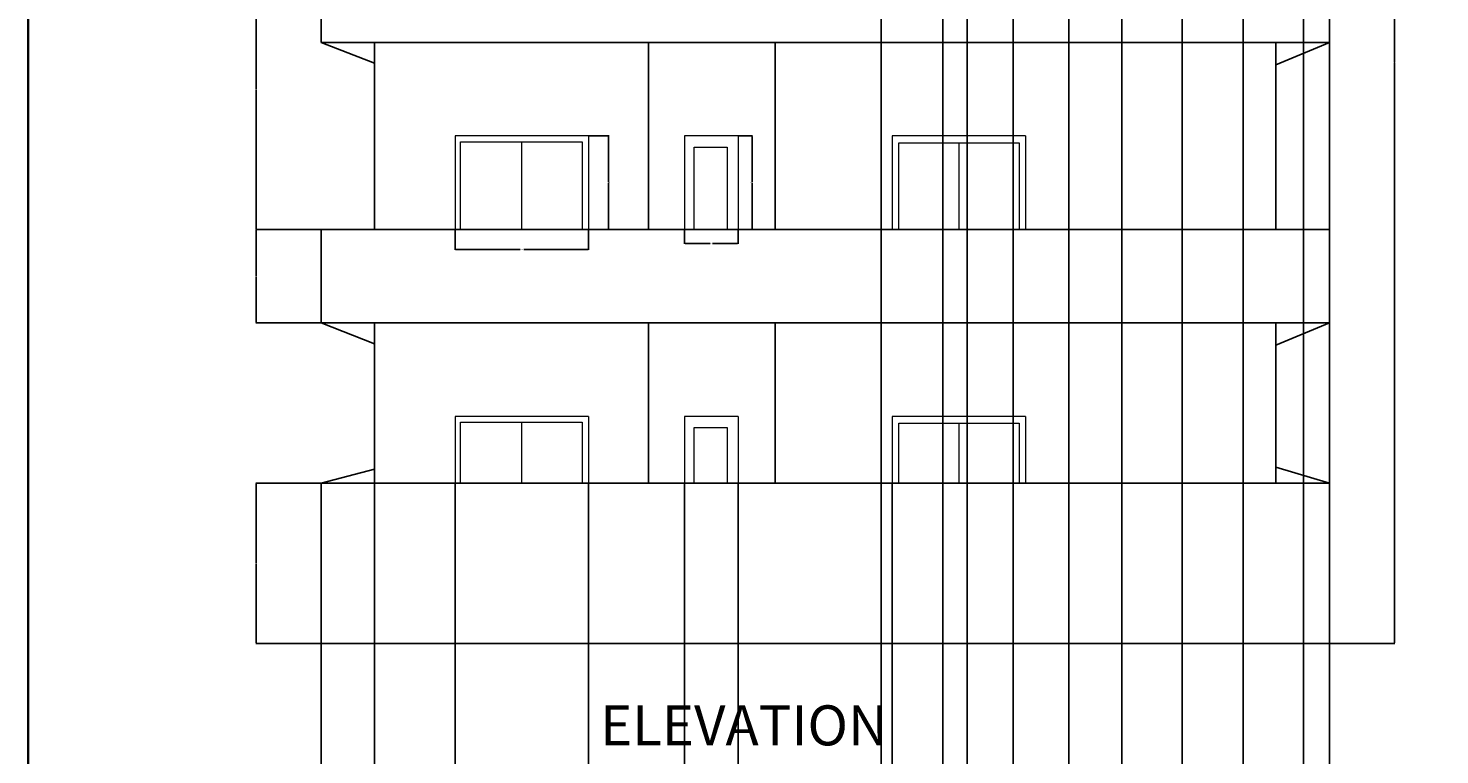
# Model space of a CAD drawing. Units: inches. Extents: x 1955 to 3324, y 980 to 3129.
# Tile 9 of 11: x 1955 to 2589, y 2488 to 2815. Entities that reach past the tile are written whole.
import ezdxf

# ---------------------------------------------------------------- set-up
doc = ezdxf.new("R2010")
doc.units = ezdxf.units.IN
for name, color, linetype, lineweight in [('A-ANNO-DIMS', 2, 'Continuous', 18), ('A-ANNO-TITL', 7, 'Continuous', 35), ('A-ANNO-TTLB', 7, 'Continuous', 35), ('A-ELEV', 7, 'Continuous', 25), ('A-GLAZ', 4, 'Continuous', 18), ('A-WALL-PATT', 252, 'Continuous', 13)]:
    doc.layers.add(name, color=color, linetype=linetype, lineweight=lineweight)
doc.styles.get("Standard").update_dxf_attribs({"font": 'arial.ttf'})
doc.dimstyles.get("Standard").update_dxf_attribs({"dimtxt": 0.18, "dimasz": 0.18, "dimexe": 0.18, "dimexo": 0.0625, "dimgap": 0.09, "dimtad": 0, "dimtih": 1, "dimtoh": 1, "dimdec": 4, "dimzin": 0, "dimdsep": 46, "dimtxsty": 'Standard', "dimcen": 0.09, "dimadec": 0, "dimazin": 0, "dimtfac": 1, "dimtdec": 4, "dimtofl": 0, "dimtmove": 0, "dimatfit": 3, "dimfxl": 1, "dimtolj": 1, "dimtzin": 0, "dimarcsym": 0})

# ---------------------------------------------------------------- blocks, each defined once
blk = doc.blocks.new('WIN-ELEV-60-L')
for p, q in [((0, 42), (0, 0)), ((60, 42), (0, 42)), ((0, 42), (0, 0)), ((60, 42), (0, 42)), ((29.78, 39.43), (29.78, 0)), ((60, 42), (60, 0)), ((60, 42), (60, 0))]:
    blk.add_line(p, q)
blk.add_lwpolyline([(2.42, 0), (2.42, 39.43), (57.15, 39.43), (57.15, 0)])
blk = doc.blocks.new('WIN-ELEV-60-R')
for p, q in [((0, 42), (0, 0)), ((60, 42), (0, 42)), ((0, 42), (0, 0)), ((60, 42), (0, 42)), ((30.07, 38.91), (30.07, 0)), ((60, 42), (60, 0)), ((60, 42), (60, 0))]:
    blk.add_line(p, q)
blk.add_lwpolyline([(3, 0), (3, 38.91), (57.15, 38.91), (57.15, 0)])
blk = doc.blocks.new('WIN-ELEV-24')
for p, q in [((0, 42), (0, 0)), ((24, 42), (0, 42)), ((0, 42), (0, 0)), ((24, 42), (0, 42)), ((24, 42), (24, 0)), ((24, 42), (24, 0))]:
    blk.add_line(p, q)
blk.add_lwpolyline([(4.32, 0), (4.32, 37), (19.12, 37), (19.12, 0)])
blk = doc.blocks.new('*D85')
at = {"layer": 'A-ANNO-DIMS', "color": 0, "lineweight": -2, "transparency": 16777216}
for p, q in [((2146.36, 2724.35), (2146.36, 2715.23)), ((2206.36, 2724.35), (2206.36, 2715.23)), ((2146.54, 2715.41), (2175.52, 2715.41)), ((2206.18, 2715.41), (2177.21, 2715.41))]:
    blk.add_line(p, q, dxfattribs=at)
at = {"layer": 'A-ANNO-DIMS', "color": 0, "transparency": 16777216}
for points in [[(2146.54, 2715.44), (2146.54, 2715.38), (2146.36, 2715.41)], [(2206.18, 2715.44), (2206.18, 2715.38), (2206.36, 2715.41)]]:
    blk.add_solid(points, dxfattribs=at)
at = {"layer": 'Defpoints', "color": 0, "transparency": 16777216}
for p in [(2146.36, 2724.41), (2206.36, 2724.41), (2206.36, 2715.41)]:
    blk.add_point(p, dxfattribs=at)
at = {"layer": 'A-ANNO-DIMS', "color": 0, "transparency": 16777216, "insert": (2176.36, 2715.41), "char_height": 0.18, "attachment_point": 5}
blk.add_mtext('\\A1;WIN. 60 TYP.', dxfattribs=at)
blk = doc.blocks.new('*D86')
at = {"layer": 'A-ANNO-DIMS', "color": 0, "lineweight": -2, "transparency": 16777216}
for p, q in [((2206.42, 2766.41), (2215.54, 2766.41)), ((2215.36, 2766.23), (2215.36, 2745.59)), ((2215.36, 2724.59), (2215.36, 2745.23)), ((2206.42, 2724.41), (2215.54, 2724.41))]:
    blk.add_line(p, q, dxfattribs=at)
at = {"layer": 'A-ANNO-DIMS', "color": 0, "transparency": 16777216}
for points in [[(2215.33, 2766.23), (2215.39, 2766.23), (2215.36, 2766.41)], [(2215.33, 2724.59), (2215.39, 2724.59), (2215.36, 2724.41)]]:
    blk.add_solid(points, dxfattribs=at)
at = {"layer": 'Defpoints', "color": 0, "transparency": 16777216}
for p in [(2206.36, 2766.41), (2215.36, 2766.41), (2206.36, 2724.41)]:
    blk.add_point(p, dxfattribs=at)
at = {"layer": 'A-ANNO-DIMS', "color": 0, "transparency": 16777216, "insert": (2215.36, 2745.41), "char_height": 0.18, "attachment_point": 5}
blk.add_mtext('\\A1;42 TYP.', dxfattribs=at)
blk = doc.blocks.new('*D89')
at = {"layer": 'A-ANNO-DIMS', "color": 0, "lineweight": -2, "transparency": 16777216}
for p, q in [((2273.55, 2766.41), (2279.97, 2766.41)), ((2279.79, 2766.23), (2279.79, 2745.59)), ((2279.79, 2724.59), (2279.79, 2745.23)), ((2273.55, 2724.41), (2279.97, 2724.41))]:
    blk.add_line(p, q, dxfattribs=at)
at = {"layer": 'A-ANNO-DIMS', "color": 0, "transparency": 16777216}
for points in [[(2279.76, 2766.23), (2279.82, 2766.23), (2279.79, 2766.41)], [(2279.76, 2724.59), (2279.82, 2724.59), (2279.79, 2724.41)]]:
    blk.add_solid(points, dxfattribs=at)
at = {"layer": 'Defpoints', "color": 0, "transparency": 16777216}
for p in [(2273.49, 2766.41), (2279.79, 2766.41), (2273.49, 2724.41)]:
    blk.add_point(p, dxfattribs=at)
at = {"layer": 'A-ANNO-DIMS', "color": 0, "transparency": 16777216, "insert": (2279.79, 2745.41), "char_height": 0.18, "attachment_point": 5}
blk.add_mtext('\\A1;WIN. 42 TYP.', dxfattribs=at)
blk = doc.blocks.new('*D90')
at = {"layer": 'A-ANNO-DIMS', "color": 0, "lineweight": -2, "transparency": 16777216}
for p, q in [((2249.49, 2724.35), (2249.49, 2717.93)), ((2273.49, 2724.35), (2273.49, 2717.93)), ((2249.67, 2718.11), (2260.96, 2718.11)), ((2273.31, 2718.11), (2262.02, 2718.11))]:
    blk.add_line(p, q, dxfattribs=at)
at = {"layer": 'A-ANNO-DIMS', "color": 0, "transparency": 16777216}
for points in [[(2249.67, 2718.14), (2249.67, 2718.08), (2249.49, 2718.11)], [(2273.31, 2718.14), (2273.31, 2718.08), (2273.49, 2718.11)]]:
    blk.add_solid(points, dxfattribs=at)
at = {"layer": 'Defpoints', "color": 0, "transparency": 16777216}
for p in [(2249.49, 2724.41), (2273.49, 2724.41), (2273.49, 2718.11)]:
    blk.add_point(p, dxfattribs=at)
at = {"layer": 'A-ANNO-DIMS', "color": 0, "transparency": 16777216, "insert": (2261.49, 2718.11), "char_height": 0.18, "attachment_point": 5}
blk.add_mtext('\\A1;24 TYP.', dxfattribs=at)
blk = doc.blocks.new('*D113')
at = {"layer": 'A-ANNO-DIMS', "color": 0, "lineweight": -2, "transparency": 16777216}
for p, q in [((2539.27, 3060.41), (2568.64, 3060.41)), ((2568.46, 3060.23), (2568.46, 2799.59)), ((2568.46, 2538.59), (2568.46, 2799.23)), ((2539.27, 2538.41), (2568.64, 2538.41))]:
    blk.add_line(p, q, dxfattribs=at)
at = {"layer": 'A-ANNO-DIMS', "color": 0, "transparency": 16777216}
for points in [[(2568.43, 3060.23), (2568.49, 3060.23), (2568.46, 3060.41)], [(2568.43, 2538.59), (2568.49, 2538.59), (2568.46, 2538.41)]]:
    blk.add_solid(points, dxfattribs=at)
at = {"layer": 'Defpoints', "color": 0, "transparency": 16777216}
for p in [(2539.21, 3060.41), (2568.46, 3060.41), (2539.21, 2538.41)]:
    blk.add_point(p, dxfattribs=at)
at = {"layer": 'A-ANNO-DIMS', "color": 0, "transparency": 16777216, "insert": (2568.46, 2799.41), "char_height": 0.18, "attachment_point": 5}
blk.add_mtext('\\A1;522', dxfattribs=at)
blk = doc.blocks.new('*D114')
at = {"layer": 'A-ANNO-DIMS', "color": 0, "lineweight": -2, "transparency": 16777216}
for p, q in [((2110.21, 2616.69), (2110.21, 2454)), ((2086.21, 2610.35), (2086.21, 2454)), ((2086.39, 2454.18), (2097.99, 2454.18)), ((2110.03, 2454.18), (2098.43, 2454.18))]:
    blk.add_line(p, q, dxfattribs=at)
at = {"layer": 'A-ANNO-DIMS', "color": 0, "transparency": 16777216}
for points in [[(2086.39, 2454.21), (2086.39, 2454.15), (2086.21, 2454.18)], [(2110.03, 2454.21), (2110.03, 2454.15), (2110.21, 2454.18)]]:
    blk.add_solid(points, dxfattribs=at)
at = {"layer": 'Defpoints', "color": 0, "transparency": 16777216}
for p in [(2110.21, 2616.75), (2086.21, 2610.41), (2110.21, 2454.18)]:
    blk.add_point(p, dxfattribs=at)
at = {"layer": 'A-ANNO-DIMS', "color": 0, "transparency": 16777216, "insert": (2098.21, 2454.18), "char_height": 0.18, "attachment_point": 5}
blk.add_mtext('\\A1;24', dxfattribs=at)
blk = doc.blocks.new('*D115')
at = {"layer": 'A-ANNO-DIMS', "color": 0, "lineweight": -2, "transparency": 16777216}
for p, q in [((2110.21, 2610.35), (2110.21, 2454)), ((2146.36, 2610.35), (2146.36, 2454)), ((2110.39, 2454.18), (2127.89, 2454.18)), ((2146.18, 2454.18), (2128.68, 2454.18))]:
    blk.add_line(p, q, dxfattribs=at)
at = {"layer": 'A-ANNO-DIMS', "color": 0, "transparency": 16777216}
for points in [[(2110.39, 2454.21), (2110.39, 2454.15), (2110.21, 2454.18)], [(2146.18, 2454.21), (2146.18, 2454.15), (2146.36, 2454.18)]]:
    blk.add_solid(points, dxfattribs=at)
at = {"layer": 'Defpoints', "color": 0, "transparency": 16777216}
for p in [(2110.21, 2610.41), (2146.36, 2610.41), (2146.36, 2454.18)]:
    blk.add_point(p, dxfattribs=at)
at = {"layer": 'A-ANNO-DIMS', "color": 0, "transparency": 16777216, "insert": (2128.29, 2454.18), "char_height": 0.18, "attachment_point": 5}
blk.add_mtext('\\A1;36.15', dxfattribs=at)
blk = doc.blocks.new('*D116')
at = {"layer": 'A-ANNO-DIMS', "color": 0, "lineweight": -2, "transparency": 16777216}
for p, q in [((2206.36, 2610.35), (2206.36, 2454)), ((2249.49, 2610.35), (2249.49, 2454)), ((2206.54, 2454.18), (2227.53, 2454.18)), ((2249.31, 2454.18), (2228.32, 2454.18))]:
    blk.add_line(p, q, dxfattribs=at)
at = {"layer": 'A-ANNO-DIMS', "color": 0, "transparency": 16777216}
for points in [[(2206.54, 2454.21), (2206.54, 2454.15), (2206.36, 2454.18)], [(2249.31, 2454.21), (2249.31, 2454.15), (2249.49, 2454.18)]]:
    blk.add_solid(points, dxfattribs=at)
at = {"layer": 'Defpoints', "color": 0, "transparency": 16777216}
for p in [(2206.36, 2610.41), (2249.49, 2610.41), (2249.49, 2454.18)]:
    blk.add_point(p, dxfattribs=at)
at = {"layer": 'A-ANNO-DIMS', "color": 0, "transparency": 16777216, "insert": (2227.93, 2454.18), "char_height": 0.18, "attachment_point": 5}
blk.add_mtext('\\A1;43.13', dxfattribs=at)
blk = doc.blocks.new('*D117')
at = {"layer": 'A-ANNO-DIMS', "color": 0, "lineweight": -2, "transparency": 16777216}
for p, q in [((2273.49, 2610.35), (2273.49, 2454)), ((2342.7, 2610.35), (2342.7, 2454)), ((2273.67, 2454.18), (2307.72, 2454.18)), ((2342.52, 2454.18), (2308.47, 2454.18))]:
    blk.add_line(p, q, dxfattribs=at)
at = {"layer": 'A-ANNO-DIMS', "color": 0, "transparency": 16777216}
for points in [[(2273.67, 2454.21), (2273.67, 2454.15), (2273.49, 2454.18)], [(2342.52, 2454.21), (2342.52, 2454.15), (2342.7, 2454.18)]]:
    blk.add_solid(points, dxfattribs=at)
at = {"layer": 'Defpoints', "color": 0, "transparency": 16777216}
for p in [(2273.49, 2610.41), (2342.7, 2610.41), (2342.7, 2454.18)]:
    blk.add_point(p, dxfattribs=at)
at = {"layer": 'A-ANNO-DIMS', "color": 0, "transparency": 16777216, "insert": (2308.09, 2454.18), "char_height": 0.18, "attachment_point": 5}
blk.add_mtext('\\A1;69.21', dxfattribs=at)
blk = doc.blocks.new('*D118')
at = {"layer": 'A-ANNO-DIMS', "color": 0, "lineweight": -2, "transparency": 16777216}
for p, q in [((2086.15, 2610.41), (2056.78, 2610.41)), ((2056.96, 2610.23), (2056.96, 2574.59)), ((2056.96, 2538.59), (2056.96, 2574.23)), ((2086.15, 2538.41), (2056.78, 2538.41))]:
    blk.add_line(p, q, dxfattribs=at)
at = {"layer": 'A-ANNO-DIMS', "color": 0, "transparency": 16777216}
for points in [[(2056.93, 2610.23), (2056.99, 2610.23), (2056.96, 2610.41)], [(2056.93, 2538.59), (2056.99, 2538.59), (2056.96, 2538.41)]]:
    blk.add_solid(points, dxfattribs=at)
at = {"layer": 'Defpoints', "color": 0, "transparency": 16777216}
for p in [(2056.96, 2610.41), (2086.21, 2610.41), (2086.21, 2538.41)]:
    blk.add_point(p, dxfattribs=at)
at = {"layer": 'A-ANNO-DIMS', "color": 0, "transparency": 16777216, "insert": (2056.96, 2574.41), "char_height": 0.18, "attachment_point": 5}
blk.add_mtext('\\A1;72', dxfattribs=at)
blk = doc.blocks.new('*D119')
at = {"layer": 'A-ANNO-DIMS', "color": 0, "lineweight": -2, "transparency": 16777216}
for p, q in [((2086.15, 2724.41), (2056.78, 2724.41)), ((2056.96, 2724.23), (2056.96, 2703.59)), ((2056.96, 2682.59), (2056.96, 2703.23)), ((2086.15, 2682.41), (2056.78, 2682.41))]:
    blk.add_line(p, q, dxfattribs=at)
at = {"layer": 'A-ANNO-DIMS', "color": 0, "transparency": 16777216}
for points in [[(2056.93, 2724.23), (2056.99, 2724.23), (2056.96, 2724.41)], [(2056.93, 2682.59), (2056.99, 2682.59), (2056.96, 2682.41)]]:
    blk.add_solid(points, dxfattribs=at)
at = {"layer": 'Defpoints', "color": 0, "transparency": 16777216}
for p in [(2056.96, 2724.41), (2086.21, 2724.41), (2086.21, 2682.41)]:
    blk.add_point(p, dxfattribs=at)
at = {"layer": 'A-ANNO-DIMS', "color": 0, "transparency": 16777216, "insert": (2056.96, 2703.41), "char_height": 0.18, "attachment_point": 5}
blk.add_mtext('\\A1;42', dxfattribs=at)
blk = doc.blocks.new('*D120')
at = {"layer": 'A-ANNO-DIMS', "color": 0, "lineweight": -2, "transparency": 16777216}
for p, q in [((2086.15, 2850.41), (2056.78, 2850.41)), ((2056.96, 2850.23), (2056.96, 2787.59)), ((2056.96, 2724.59), (2056.96, 2787.23)), ((2086.15, 2724.41), (2056.78, 2724.41))]:
    blk.add_line(p, q, dxfattribs=at)
at = {"layer": 'A-ANNO-DIMS', "color": 0, "transparency": 16777216}
for points in [[(2056.93, 2850.23), (2056.99, 2850.23), (2056.96, 2850.41)], [(2056.93, 2724.59), (2056.99, 2724.59), (2056.96, 2724.41)]]:
    blk.add_solid(points, dxfattribs=at)
at = {"layer": 'Defpoints', "color": 0, "transparency": 16777216}
for p in [(2056.96, 2850.41), (2086.21, 2850.41), (2086.21, 2724.41)]:
    blk.add_point(p, dxfattribs=at)
at = {"layer": 'A-ANNO-DIMS', "color": 0, "transparency": 16777216, "insert": (2056.96, 2787.41), "char_height": 0.18, "attachment_point": 5}
blk.add_mtext('\\A1;126', dxfattribs=at)
blk = doc.blocks.new('*D123')
at = {"layer": 'A-ANNO-DIMS', "color": 0, "lineweight": -2, "transparency": 16777216}
for p, q in [((2337.77, 3041.34), (2337.77, 2454)), ((2365.46, 3041.34), (2365.46, 2454)), ((2337.95, 2454.18), (2351.22, 2454.18)), ((2365.28, 2454.18), (2352.01, 2454.18))]:
    blk.add_line(p, q, dxfattribs=at)
at = {"layer": 'A-ANNO-DIMS', "color": 0, "transparency": 16777216}
for points in [[(2337.95, 2454.21), (2337.95, 2454.15), (2337.77, 2454.18)], [(2365.28, 2454.21), (2365.28, 2454.15), (2365.46, 2454.18)]]:
    blk.add_solid(points, dxfattribs=at)
at = {"layer": 'Defpoints', "color": 0, "transparency": 16777216}
for p in [(2337.77, 3041.4), (2365.46, 3041.4), (2365.46, 2454.18)]:
    blk.add_point(p, dxfattribs=at)
at = {"layer": 'A-ANNO-DIMS', "color": 0, "transparency": 16777216, "insert": (2351.62, 2454.18), "char_height": 0.18, "attachment_point": 5}
blk.add_mtext('\\A1;27.69', dxfattribs=at)
blk = doc.blocks.new('*D124')
at = {"layer": 'A-ANNO-DIMS', "color": 0, "lineweight": -2, "transparency": 16777216}
for p, q in [((2376.45, 2978.61), (2376.45, 2454)), ((2397.08, 2978.61), (2397.08, 2454)), ((2376.63, 2454.18), (2386.37, 2454.18)), ((2396.9, 2454.18), (2387.16, 2454.18))]:
    blk.add_line(p, q, dxfattribs=at)
at = {"layer": 'A-ANNO-DIMS', "color": 0, "transparency": 16777216}
for points in [[(2376.63, 2454.21), (2376.63, 2454.15), (2376.45, 2454.18)], [(2396.9, 2454.21), (2396.9, 2454.15), (2397.08, 2454.18)]]:
    blk.add_solid(points, dxfattribs=at)
at = {"layer": 'Defpoints', "color": 0, "transparency": 16777216}
for p in [(2376.45, 2978.67), (2397.08, 2978.67), (2397.08, 2454.18)]:
    blk.add_point(p, dxfattribs=at)
at = {"layer": 'A-ANNO-DIMS', "color": 0, "transparency": 16777216, "insert": (2386.76, 2454.18), "char_height": 0.18, "attachment_point": 5}
blk.add_mtext('\\A1;20.63', dxfattribs=at)
blk = doc.blocks.new('*D125')
at = {"layer": 'A-ANNO-DIMS', "color": 0, "lineweight": -2, "transparency": 16777216}
for p, q in [((2397.08, 2978.61), (2397.08, 2454)), ((2422.2, 2978.61), (2422.2, 2454)), ((2397.26, 2454.18), (2409.24, 2454.18)), ((2422.02, 2454.18), (2410.03, 2454.18))]:
    blk.add_line(p, q, dxfattribs=at)
at = {"layer": 'A-ANNO-DIMS', "color": 0, "transparency": 16777216}
for points in [[(2397.26, 2454.21), (2397.26, 2454.15), (2397.08, 2454.18)], [(2422.02, 2454.21), (2422.02, 2454.15), (2422.2, 2454.18)]]:
    blk.add_solid(points, dxfattribs=at)
at = {"layer": 'Defpoints', "color": 0, "transparency": 16777216}
for p in [(2397.08, 2978.67), (2422.2, 2978.67), (2422.2, 2454.18)]:
    blk.add_point(p, dxfattribs=at)
at = {"layer": 'A-ANNO-DIMS', "color": 0, "transparency": 16777216, "insert": (2409.64, 2454.18), "char_height": 0.18, "attachment_point": 5}
blk.add_mtext('\\A1;25.12', dxfattribs=at)
blk = doc.blocks.new('*D126')
at = {"layer": 'A-ANNO-DIMS', "color": 0, "lineweight": -2, "transparency": 16777216}
for p, q in [((2422.2, 2978.61), (2422.2, 2454)), ((2445.92, 2978.61), (2445.92, 2454)), ((2422.38, 2454.18), (2433.59, 2454.18)), ((2445.74, 2454.18), (2434.52, 2454.18))]:
    blk.add_line(p, q, dxfattribs=at)
at = {"layer": 'A-ANNO-DIMS', "color": 0, "transparency": 16777216}
for points in [[(2422.38, 2454.21), (2422.38, 2454.15), (2422.2, 2454.18)], [(2445.74, 2454.21), (2445.74, 2454.15), (2445.92, 2454.18)]]:
    blk.add_solid(points, dxfattribs=at)
at = {"layer": 'Defpoints', "color": 0, "transparency": 16777216}
for p in [(2422.2, 2978.67), (2445.92, 2978.67), (2445.92, 2454.18)]:
    blk.add_point(p, dxfattribs=at)
at = {"layer": 'A-ANNO-DIMS', "color": 0, "transparency": 16777216, "insert": (2434.06, 2454.18), "char_height": 0.18, "attachment_point": 5}
blk.add_mtext('\\A1;23.727', dxfattribs=at)
blk = doc.blocks.new('*D127')
at = {"layer": 'A-ANNO-DIMS', "color": 0, "lineweight": -2, "transparency": 16777216}
for p, q in [((2445.92, 2978.61), (2445.92, 2454)), ((2473.12, 2978.61), (2473.12, 2454)), ((2446.1, 2454.18), (2459.05, 2454.18)), ((2472.94, 2454.18), (2459.99, 2454.18))]:
    blk.add_line(p, q, dxfattribs=at)
at = {"layer": 'A-ANNO-DIMS', "color": 0, "transparency": 16777216}
for points in [[(2446.1, 2454.21), (2446.1, 2454.15), (2445.92, 2454.18)], [(2472.94, 2454.21), (2472.94, 2454.15), (2473.12, 2454.18)]]:
    blk.add_solid(points, dxfattribs=at)
at = {"layer": 'Defpoints', "color": 0, "transparency": 16777216}
for p in [(2445.92, 2978.67), (2473.12, 2978.67), (2473.12, 2454.18)]:
    blk.add_point(p, dxfattribs=at)
at = {"layer": 'A-ANNO-DIMS', "color": 0, "transparency": 16777216, "insert": (2459.52, 2454.18), "char_height": 0.18, "attachment_point": 5}
blk.add_mtext('\\A1;27.195', dxfattribs=at)
blk = doc.blocks.new('*D128')
at = {"layer": 'A-ANNO-DIMS', "color": 0, "lineweight": -2, "transparency": 16777216}
for p, q in [((2473.12, 2978.61), (2473.12, 2454)), ((2500.43, 2978.61), (2500.43, 2454)), ((2473.3, 2454.18), (2486.31, 2454.18)), ((2500.25, 2454.18), (2487.24, 2454.18))]:
    blk.add_line(p, q, dxfattribs=at)
at = {"layer": 'A-ANNO-DIMS', "color": 0, "transparency": 16777216}
for points in [[(2473.3, 2454.21), (2473.3, 2454.15), (2473.12, 2454.18)], [(2500.25, 2454.21), (2500.25, 2454.15), (2500.43, 2454.18)]]:
    blk.add_solid(points, dxfattribs=at)
at = {"layer": 'Defpoints', "color": 0, "transparency": 16777216}
for p in [(2473.12, 2978.67), (2500.43, 2978.67), (2500.43, 2454.18)]:
    blk.add_point(p, dxfattribs=at)
at = {"layer": 'A-ANNO-DIMS', "color": 0, "transparency": 16777216, "insert": (2486.77, 2454.18), "char_height": 0.18, "attachment_point": 5}
blk.add_mtext('\\A1;27.314', dxfattribs=at)
blk = doc.blocks.new('*D129')
at = {"layer": 'A-ANNO-DIMS', "color": 0, "lineweight": -2, "transparency": 16777216}
for p, q in [((2500.43, 2978.61), (2500.43, 2454)), ((2527.66, 2978.61), (2527.66, 2454)), ((2500.61, 2454.18), (2513.65, 2454.18)), ((2527.48, 2454.18), (2514.44, 2454.18))]:
    blk.add_line(p, q, dxfattribs=at)
at = {"layer": 'A-ANNO-DIMS', "color": 0, "transparency": 16777216}
for points in [[(2500.61, 2454.21), (2500.61, 2454.15), (2500.43, 2454.18)], [(2527.48, 2454.21), (2527.48, 2454.15), (2527.66, 2454.18)]]:
    blk.add_solid(points, dxfattribs=at)
at = {"layer": 'Defpoints', "color": 0, "transparency": 16777216}
for p in [(2500.43, 2978.67), (2527.66, 2978.67), (2527.66, 2454.18)]:
    blk.add_point(p, dxfattribs=at)
at = {"layer": 'A-ANNO-DIMS', "color": 0, "transparency": 16777216, "insert": (2514.05, 2454.18), "char_height": 0.18, "attachment_point": 5}
blk.add_mtext('\\A1;27.23', dxfattribs=at)
blk = doc.blocks.new('*D130')
at = {"layer": 'A-ANNO-DIMS', "color": 0, "lineweight": -2, "transparency": 16777216}
for p, q in [((2539.21, 3060.35), (2539.21, 2454)), ((2527.66, 3047.91), (2527.66, 2454)), ((2527.84, 2454.18), (2533.05, 2454.18)), ((2539.03, 2454.18), (2533.82, 2454.18))]:
    blk.add_line(p, q, dxfattribs=at)
at = {"layer": 'A-ANNO-DIMS', "color": 0, "transparency": 16777216}
for points in [[(2527.84, 2454.21), (2527.84, 2454.15), (2527.66, 2454.18)], [(2539.03, 2454.21), (2539.03, 2454.15), (2539.21, 2454.18)]]:
    blk.add_solid(points, dxfattribs=at)
at = {"layer": 'Defpoints', "color": 0, "transparency": 16777216}
for p in [(2539.21, 3060.41), (2527.66, 3047.98), (2539.21, 2454.18)]:
    blk.add_point(p, dxfattribs=at)
at = {"layer": 'A-ANNO-DIMS', "color": 0, "transparency": 16777216, "insert": (2533.44, 2454.18), "char_height": 0.18, "attachment_point": 5}
blk.add_mtext('\\A1;11.55', dxfattribs=at)

msp = doc.modelspace()

# ---------------------------------------------------------------- hatches: boundary and pattern name
at = {"layer": 'A-WALL-PATT'}
h = msp.add_hatch(dxfattribs=at)
h.set_pattern_fill('ANSI32', color=256)
h.paths.add_polyline_path([(2361.4775, 2456.5037), (2270.2755, 2456.5037), (2270.2755, 2447.5037), (2285.7102, 2447.5037), (2285.7102, 2363.5037), (2281.1795, 2363.5037), (2281.1795, 2359.0037), (2290.2102, 2359.0037), (2290.2102, 2447.5037), (2361.4775, 2447.5037), (2361.4775, 2452.0037)])
h.paths.add_polyline_path([(2246.2755, 2456.5037), (2197.6809, 2456.5037), (2197.6809, 2447.5037), (2233.2102, 2447.5037), (2233.2102, 2355.6044), (2237.7102, 2355.6044), (2237.7102, 2447.5037), (2246.2755, 2447.5037)], flags=17)
h.paths.add_polyline_path([(2137.6809, 2456.5037), (2110.2102, 2456.5037), (2110.2102, 2312.5037), (2152.2102, 2312.5037), (2281.2102, 2312.5037), (2281.2102, 2107.6185), (2290.2102, 2107.6185), (2290.2102, 2267.9289), (2329.216, 2267.9289), (2329.216, 2272.4289), (2329.216, 2276.9289), (2290.2102, 2276.9289), (2290.2102, 2321.5037), (2281.2102, 2321.5037), (2119.2102, 2321.5037), (2119.2102, 2447.5037), (2137.6809, 2447.5037)])
h.paths.add_polyline_path([(2515.2102, 2456.5037), (2421.4775, 2456.5037), (2421.4775, 2447.5037), (2506.2102, 2447.5037), (2506.2102, 2415.6626), (2515.2102, 2415.6626)])
h.paths.add_polyline_path([(2515.2102, 2355.6626), (2506.2102, 2355.6626), (2506.2102, 2321.5037), (2424.9282, 2321.5037), (2424.9282, 2312.5037), (2461.2102, 2312.5037), (2470.2102, 2312.5037), (2515.2102, 2312.5037)])
h.paths.add_polyline_path([(2515.2102, 2232.5037), (2470.2102, 2232.5037), (2470.2102, 2237.3759), (2465.7102, 2237.3759), (2461.2102, 2237.3759), (2461.2102, 2232.5037), (2377.2219, 2232.5037), (2377.2219, 2321.5037), (2368.2219, 2321.5037), (2368.2219, 2276.9289), (2359.3802, 2276.9289), (2359.3802, 2272.4289), (2359.3802, 2267.9289), (2368.2219, 2267.9289), (2368.2219, 2223.5037), (2377.2219, 2223.5037), (2461.2102, 2223.5037), (2506.2102, 2223.5037), (2506.2102, 2129.5037), (2461.2102, 2129.5037), (2387.2102, 2129.5037), (2368.2219, 2129.5037), (2368.2219, 2056.4936), (2361.0095, 2056.4936), (2361.0095, 2051.9936), (2361.0095, 2047.4936), (2368.2219, 2047.4936), (2368.2219, 2031.5037), (2377.2219, 2031.5037), (2377.2219, 2120.5037), (2461.2102, 2120.5037), (2461.2102, 2112.7921), (2470.2102, 2112.7921), (2470.2102, 2120.5037), (2515.2102, 2120.5037), (2515.2102, 2129.5037)])
h.paths.add_polyline_path([(2470.2102, 2277.1758), (2461.2102, 2277.1758), (2461.2102, 2272.5037), (2461.2102, 2270.2549), (2470.2102, 2270.2549), (2470.2102, 2272.5037)], flags=17)
h.paths.add_polyline_path([(2515.2102, 2040.5037), (2470.2102, 2040.5037), (2417.8264, 2040.5037), (2417.8264, 2031.5037), (2506.2102, 2031.5037), (2506.2102, 2005.3639), (2515.2102, 2005.3639)])
h.paths.add_polyline_path([(2506.2102, 1905.5037), (2402.6963, 1905.5037), (2402.6963, 1896.5037), (2506.2102, 1896.5037)])
h.paths.add_polyline_path([(2515.2102, 1945.3639), (2506.2102, 1945.3639), (2506.2102, 1905.5037), (2506.2102, 1896.5037), (2515.2102, 1896.5037)])
h.paths.add_polyline_path([(2342.6963, 1901.0037), (2342.6963, 1905.5037), (2273.4892, 1905.5037), (2273.4892, 1896.5037), (2342.6963, 1896.5037)])
h.paths.add_polyline_path([(2290.2102, 1994.0037), (2283.612, 1994.0037), (2283.612, 1991.7537), (2283.612, 1989.5037), (2285.7102, 1989.5037), (2285.7102, 1905.5037), (2290.2102, 1905.5037)])
h.paths.add_polyline_path([(2249.4892, 1905.5037), (2237.7102, 1905.5037), (2206.3617, 1905.5037), (2206.3617, 1896.5037), (2249.4892, 1896.5037), (2249.4892, 1901.0037)])
h.paths.add_polyline_path([(2237.7102, 1989.5037), (2261.7102, 1989.5037), (2261.7102, 1994.0037), (2237.7102, 1994.0037), (2237.7102, 1999.266), (2235.4602, 1999.266), (2233.2102, 1999.266), (2233.2102, 1994.0037), (2233.2102, 1905.5037), (2237.7102, 1905.5037)])
h.paths.add_polyline_path([(2119.2102, 1947.5144), (2110.2102, 1947.5144), (2110.2102, 1896.5037), (2119.2102, 1896.5037), (2146.3617, 1896.5037), (2146.3617, 1901.0037), (2146.3617, 1905.5037), (2119.2102, 1905.5037)])
h.paths.add_polyline_path([(2119.2102, 2068.6379), (2110.2102, 2068.6379), (2110.2102, 2007.5144), (2119.2102, 2007.5144), (2119.2102, 2031.5037), (2233.2102, 2031.5037), (2233.2102, 2027.9287), (2235.4602, 2027.9287), (2237.7102, 2027.9287), (2237.7102, 2031.5037), (2281.2102, 2031.5037), (2290.2102, 2031.5037), (2290.2102, 2047.4936), (2326.409, 2047.4936), (2326.409, 2056.4936), (2290.2102, 2056.4936), (2290.2102, 2071.2722), (2285.7102, 2071.2722), (2281.2102, 2071.2722), (2281.2102, 2040.5037), (2227.2102, 2040.5037), (2227.2102, 2111.2571), (2222.7102, 2111.2571), (2218.2102, 2111.2571), (2218.2102, 2040.5037), (2119.2102, 2040.5037)])
h.paths.add_polyline_path([(2236.9166, 2214.5037), (2161.2102, 2214.5037), (2161.2102, 2221.6488), (2152.2102, 2221.6488), (2152.2102, 2214.5037), (2110.2102, 2214.5037), (2110.2102, 2205.5037), (2131.2394, 2205.5037), (2131.2394, 2198.3478), (2140.2394, 2198.3478), (2140.2394, 2205.5037), (2224.2394, 2205.5037), (2224.2394, 2200.2317), (2228.7394, 2200.2317), (2233.2394, 2200.2317), (2233.2394, 2205.5037), (2236.9166, 2205.5037)], flags=17)
h.paths.add_polyline_path([(2236.9166, 2157.5037), (2233.2394, 2157.5037), (2233.2394, 2178.9172), (2228.7394, 2178.9172), (2224.2394, 2178.9172), (2224.2394, 2157.5037), (2140.2394, 2157.5037), (2140.2394, 2174.3478), (2131.2394, 2174.3478), (2131.2394, 2157.5037), (2110.2102, 2157.5037), (2110.2102, 2128.6379), (2119.2102, 2128.6379), (2119.2102, 2148.5037), (2218.2102, 2148.5037), (2218.2102, 2141.7262), (2222.7102, 2141.7262), (2227.2102, 2141.7262), (2227.2102, 2148.5037), (2236.9166, 2148.5037)], flags=0)
h.paths.add_polyline_path([(3084.7449, 2537.3808), (3212.7954, 2537.3808), (3212.7954, 2555.9271), (3084.7449, 2555.9271)], flags=9)
h.paths.add_polyline_path([(3068.7485, 2853.43), (3169.977, 2853.43), (3169.977, 2871.9764), (3068.7485, 2871.9764)], flags=9)
h.paths.add_polyline_path([(3074.1798, 2918.0252), (3126.4732, 2918.0252), (3126.4732, 2936.5716), (3074.1798, 2936.5716)], flags=9)
h.paths.add_polyline_path([(3073.0928, 2947.3127), (3199.0499, 2947.3127), (3199.0499, 2965.8591), (3073.0928, 2965.8591)], flags=9)
h.paths.add_polyline_path([(2733.8393, 2484.8678), (2879.7915, 2484.8678), (2879.7915, 2521.9606), (2733.8393, 2521.9606)], flags=9)
h.paths.add_polyline_path([(2204.9881, 2482.4168), (2355.1272, 2482.4168), (2355.1272, 2519.5095), (2204.9881, 2519.5095)], flags=9)
h.paths.add_polyline_path([(3062.1429, 2387.2466), (3079.3735, 2387.2466), (3079.3735, 2411.9751), (3062.1429, 2411.9751)], flags=9)
h.paths.add_polyline_path([(2190.1574, 2158.8439), (2219.315, 2158.8439), (2219.315, 2177.5013), (2190.1574, 2177.5013)], flags=25)
h.paths.add_polyline_path([(2213.6766, 1840.7276), (2405.0382, 1840.7276), (2405.0382, 1865.4561), (2213.6766, 1865.4561)], flags=9)
h.paths.add_polyline_path([(2180.5398, 2233.911), (2213.9471, 2233.911), (2213.9471, 2252.5683), (2180.5398, 2252.5683)], flags=25)
h.paths.add_polyline_path([(2134.4484, 2238.3973), (2134.4484, 2274.2807), (2115.791, 2274.2807), (2115.791, 2238.3973)], flags=25)
h.paths.add_polyline_path([(2135.1593, 2122.9991), (2173.7507, 2122.9991), (2173.7507, 2141.6565), (2135.1593, 2141.6565)], flags=25)
h.paths.add_polyline_path([(2129.8822, 2002.1912), (2168.4736, 2002.1912), (2168.4736, 2020.8486), (2129.8822, 2020.8486)], flags=9)
h.paths.add_polyline_path([(2239.6647, 1953.4107), (2268.8973, 1953.4107), (2268.8973, 1972.068), (2239.6647, 1972.068)], flags=9)
h.paths.add_polyline_path([(2352.8562, 1951.2904), (2402.1775, 1951.2904), (2402.1775, 1969.9477), (2352.8562, 1969.9477)], flags=9)
h.paths.add_polyline_path([(2500.1358, 2055.32), (2500.1358, 2091.2034), (2481.4784, 2091.2034), (2481.4784, 2055.32)], flags=25)
h.paths.add_polyline_path([(2391.2702, 2058.6821), (2424.4285, 2058.6821), (2424.4285, 2077.3394), (2391.2702, 2077.3394)], flags=25)
h.paths.add_polyline_path([(2507.7996, 2257.2758), (2507.7996, 2293.1592), (2489.1422, 2293.1592), (2489.1422, 2257.2758)], flags=25)
h.paths.add_polyline_path([(2386.8349, 2273.8734), (2419.9931, 2273.8734), (2419.9931, 2292.5307), (2386.8349, 2292.5307)], flags=25)
h.paths.add_polyline_path([(2335.374, 2373.3267), (2384.6953, 2373.3267), (2384.6953, 2391.984), (2335.374, 2391.984)], flags=9)
h.paths.add_polyline_path([(2243.8205, 2380.6539), (2273.0531, 2380.6539), (2273.0531, 2399.3113), (2243.8205, 2399.3113)], flags=25)
h.paths.add_polyline_path([(2126.2627, 2321.6894), (2164.8541, 2321.6894), (2164.8541, 2340.3467), (2126.2627, 2340.3467)], flags=25)

# ---------------------------------------------------------------- linework, layer by layer
at = {"layer": 'A-ANNO-TTLB'}
msp.add_lwpolyline([(1954.5391, 3128.9103), (3323.9705, 3128.9103), (3323.9705, 1703.6826), (1954.5391, 1703.6826)], close=True, dxfattribs=at)
at = {"layer": 'A-ELEV'}
for p, q in [((2086.2102, 2808.4103), (2086.2102, 2850.4103)), ((2539.2102, 2808.4103), (2539.2102, 2850.4103)), ((2539.2102, 2808.4103), (2086.2102, 2808.4103)), ((2086.2102, 2808.4103), (2110.2102, 2799.0754)), ((2110.2102, 2808.4103), (2110.2102, 2724.4103)), ((2110.2102, 2808.4103), (2110.2102, 2790.4103)), ((2233.2102, 2808.4103), (2233.2102, 2724.4103)), ((2290.2102, 2808.4103), (2290.2102, 2724.4103)), ((2515.2102, 2808.4103), (2515.2102, 2724.4103)), ((2539.2102, 2808.4103), (2515.2102, 2798.3558)), ((2515.2102, 2808.4103), (2515.2102, 2790.4103)), ((2539.2102, 2724.4103), (2086.2102, 2724.4103)), ((2086.2102, 2682.4103), (2086.2102, 2724.4103)), ((2539.2102, 2682.4103), (2539.2102, 2724.4103)), ((2539.2102, 2682.4103), (2086.2102, 2682.4103)), ((2086.2102, 2682.4103), (2110.2102, 2673.0754)), ((2110.2102, 2682.4103), (2110.2102, 2610.4103)), ((2110.2102, 2682.4103), (2110.2102, 2664.4103)), ((2233.2102, 2682.4103), (2233.2102, 2610.4103)), ((2290.2102, 2682.4103), (2290.2102, 2610.4103)), ((2515.2102, 2682.4103), (2515.2102, 2610.4103)), ((2539.2102, 2682.4103), (2515.2102, 2672.3558)), ((2515.2102, 2682.4103), (2515.2102, 2664.4103)), ((2086.2102, 2610.4103), (2110.2102, 2616.7505)), ((2110.2102, 2616.7505), (2110.2102, 2616.7505)), ((2539.2102, 2610.4103), (2515.2102, 2617.5927)), ((2110.2102, 2610.4103), (2086.2102, 2610.4103)), ((2086.2102, 2610.4103), (2086.2102, 2538.4103)), ((2539.2102, 2610.4103), (2110.2102, 2610.4103)), ((2539.2102, 2538.4103), (2539.2102, 2610.4103)), ((2086.2102, 2538.4103), (2110.2102, 2538.4103)), ((2515.2102, 2538.4103), (2110.2102, 2538.4103)), ((2515.2102, 2538.4103), (2539.2102, 2538.4103))]:
    msp.add_line(p, q, dxfattribs=at)
at = {"layer": 'A-GLAZ'}
for p, q in [((2146.3617, 2640.4103), (2146.3617, 2610.4103)), ((2206.3617, 2640.4103), (2146.3617, 2640.4103)), ((2206.3617, 2640.4103), (2206.3617, 2610.4103)), ((2249.4892, 2640.4103), (2249.4892, 2610.4103)), ((2273.4892, 2640.4103), (2249.4892, 2640.4103)), ((2273.4892, 2640.4103), (2273.4892, 2610.4103)), ((2342.6963, 2640.4103), (2342.6963, 2610.4103)), ((2402.6963, 2640.4103), (2342.6963, 2640.4103)), ((2402.6963, 2640.4103), (2402.6963, 2610.4103)), ((2176.1429, 2637.8369), (2176.1429, 2610.4103)), ((2372.7704, 2637.3248), (2372.7704, 2610.4103))]:
    msp.add_line(p, q, dxfattribs=at)
for points in [[(2148.7779, 2610.4103), (2148.7779, 2637.8369), (2203.5079, 2637.8369), (2203.5079, 2610.4103)], [(2253.8115, 2610.4103), (2253.8115, 2635.414), (2268.6108, 2635.414), (2268.6108, 2610.4103)], [(2345.6923, 2610.4103), (2345.6923, 2637.3248), (2399.8485, 2637.3248), (2399.8485, 2610.4103)]]:
    msp.add_lwpolyline(points, dxfattribs=at)

# ---------------------------------------------------------------- block references
for name, p in [('WIN-ELEV-60-L', (2146.362, 2724.41)), ('WIN-ELEV-24', (2249.489, 2724.41)), ('WIN-ELEV-60-R', (2342.696, 2724.41))]:
    msp.add_blockref(name, p, dxfattribs=at)

# ---------------------------------------------------------------- texts
at = {"layer": 'A-ANNO-TITL', "insert": (2211.4771, 2510.5648), "char_height": 18, "attachment_point": 1}
msp.add_mtext_dynamic_manual_height_columns('ELEVATION', width=383.628381, gutter_width=12.5, heights=[0], dxfattribs=at)

# ---------------------------------------------------------------- dimensions: what is measured, and where the dimension line sits
at = {"layer": 'A-ANNO-DIMS'}
for base, p1, p2, override, picture, middle in [((2539.2102, 2454.185), (2527.661, 3047.9754), (2539.2102, 3060.4103), {"dimdec": 2, "dimlfac": 1, "dimrnd": 0, "dimzin": 0, "dimdsep": 46, "dimlunit": 2}, '*D130', (2533.4356, 2454.185)), ((2365.4619, 2454.185), (2337.7695, 3041.4019), (2365.4619, 3041.4019), {"dimdec": 2, "dimlfac": 1, "dimrnd": 0, "dimzin": 0, "dimdsep": 46, "dimlunit": 2}, '*D123', (2351.6157, 2454.185)), ((2397.0773, 2454.185), (2376.4478, 2978.6742), (2397.0773, 2978.6742), {"dimdec": 2, "dimlfac": 1, "dimrnd": 0, "dimzin": 0, "dimdsep": 46, "dimlunit": 2}, '*D124', (2386.7626, 2454.185)), ((2422.1951, 2454.185), (2397.0773, 2978.6742), (2422.1951, 2978.6742), {"dimdec": 2, "dimlfac": 1, "dimrnd": 0, "dimzin": 0, "dimdsep": 46, "dimlunit": 2}, '*D125', (2409.6362, 2454.185)), ((2445.9223, 2454.185), (2422.1951, 2978.6742), (2445.9223, 2978.6742), {"dimdec": 3, "dimlfac": 1, "dimrnd": 0, "dimzin": 0, "dimdsep": 46, "dimlunit": 2}, '*D126', (2434.0587, 2454.185)), ((2473.1169, 2454.185), (2445.9223, 2978.6742), (2473.1169, 2978.6742), {"dimdec": 3, "dimlfac": 1, "dimrnd": 0, "dimzin": 0, "dimdsep": 46, "dimlunit": 2}, '*D127', (2459.5196, 2454.185)), ((2500.4308, 2454.185), (2473.1169, 2978.6742), (2500.4308, 2978.6742), {"dimdec": 3, "dimlfac": 1, "dimrnd": 0, "dimzin": 0, "dimdsep": 46, "dimlunit": 2}, '*D128', (2486.7738, 2454.185)), ((2527.661, 2454.185), (2500.4308, 2978.6742), (2527.661, 2978.6742), {"dimdec": 2, "dimlfac": 1, "dimrnd": 0, "dimzin": 0, "dimdsep": 46, "dimlunit": 2}, '*D129', (2514.0459, 2454.185)), ((2110.2102, 2454.185), (2086.2102, 2610.4103), (2110.2102, 2616.7505), {"dimdec": 0, "dimlfac": 1, "dimrnd": 0, "dimzin": 0, "dimdsep": 46, "dimlunit": 2}, '*D114', (2098.2102, 2454.185)), ((2146.3617, 2454.185), (2110.2102, 2610.4103), (2146.3617, 2610.4103), {"dimdec": 2, "dimlfac": 1, "dimrnd": 0, "dimzin": 0, "dimdsep": 46, "dimlunit": 2}, '*D115', (2128.286, 2454.185)), ((2249.4892, 2454.185), (2206.3617, 2610.4103), (2249.4892, 2610.4103), {"dimdec": 2, "dimlfac": 1, "dimrnd": 0, "dimzin": 0, "dimdsep": 46, "dimlunit": 2}, '*D116', (2227.9254, 2454.185)), ((2342.6963, 2454.185), (2273.4892, 2610.4103), (2342.6963, 2610.4103), {"dimdec": 2, "dimlfac": 1, "dimrnd": 0, "dimzin": 0, "dimdsep": 46, "dimlunit": 2}, '*D117', (2308.0927, 2454.185))]:
    dim = msp.add_linear_dim(base=base, p1=p1, p2=p2, dimstyle='Standard', override=override, dxfattribs=at)
    dim.commit()
    dim.dimension.update_dxf_attribs({"geometry": picture, "text_midpoint": middle})
for base, p1, p2, picture, middle in [((2568.4602, 3060.4103), (2539.2102, 2538.4103), (2539.2102, 3060.4103), '*D113', (2568.4602, 2799.4103)), ((2056.9602, 2850.4103), (2086.2102, 2724.4103), (2086.2102, 2850.4103), '*D120', (2056.9602, 2787.4103)), ((2056.9602, 2724.4103), (2086.2102, 2682.4103), (2086.2102, 2724.4103), '*D119', (2056.9602, 2703.4103)), ((2056.9602, 2610.4103), (2086.2102, 2538.4103), (2086.2102, 2610.4103), '*D118', (2056.9602, 2574.4103))]:
    dim = msp.add_linear_dim(base=base, p1=p1, p2=p2, angle=90, dimstyle='Standard', override={"dimdec": 0, "dimlfac": 1, "dimrnd": 0, "dimzin": 0, "dimdsep": 46, "dimlunit": 2}, dxfattribs=at)
    dim.commit()
    dim.dimension.update_dxf_attribs({"geometry": picture, "text_midpoint": middle})
for base, p1, p2, text, picture, middle in [((2215.3617, 2766.4103), (2206.3617, 2724.4103), (2206.3617, 2766.4103), '<> TYP.', '*D86', (2215.3617, 2745.4103)), ((2279.7892, 2766.4103), (2273.4892, 2724.4103), (2273.4892, 2766.4103), 'WIN. <> TYP.', '*D89', (2279.7892, 2745.4103))]:
    dim = msp.add_linear_dim(base=base, p1=p1, p2=p2, angle=90, text=text, dimstyle='Standard', override={"dimdec": 0, "dimlfac": 1, "dimrnd": 0, "dimzin": 0, "dimdsep": 46, "dimlunit": 2}, dxfattribs=at)
    dim.commit()
    dim.dimension.update_dxf_attribs({"geometry": picture, "text_midpoint": middle})
for base, p1, p2, text, picture, middle in [((2206.3617, 2715.4103), (2146.3617, 2724.4103), (2206.3617, 2724.4103), 'WIN. <> TYP.', '*D85', (2176.3617, 2715.4103)), ((2273.4892, 2718.1103), (2249.4892, 2724.4103), (2273.4892, 2724.4103), '<> TYP.', '*D90', (2261.4892, 2718.1103))]:
    dim = msp.add_linear_dim(base=base, p1=p1, p2=p2, text=text, dimstyle='Standard', override={"dimdec": 0, "dimlfac": 1, "dimrnd": 0, "dimzin": 0, "dimdsep": 46, "dimlunit": 2}, dxfattribs=at)
    dim.commit()
    dim.dimension.update_dxf_attribs({"geometry": picture, "text_midpoint": middle})

doc.saveas('drawing.dxf')
